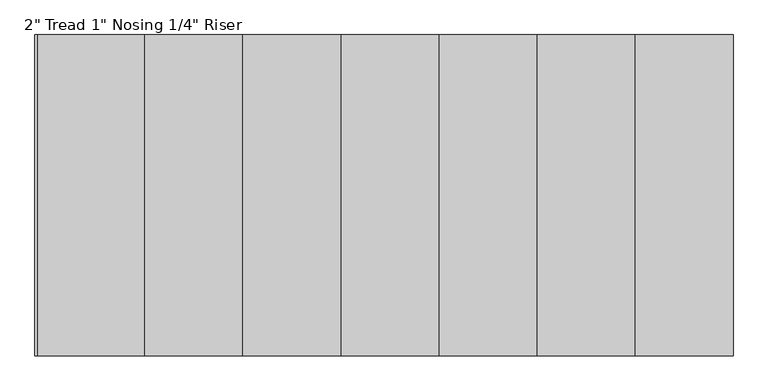
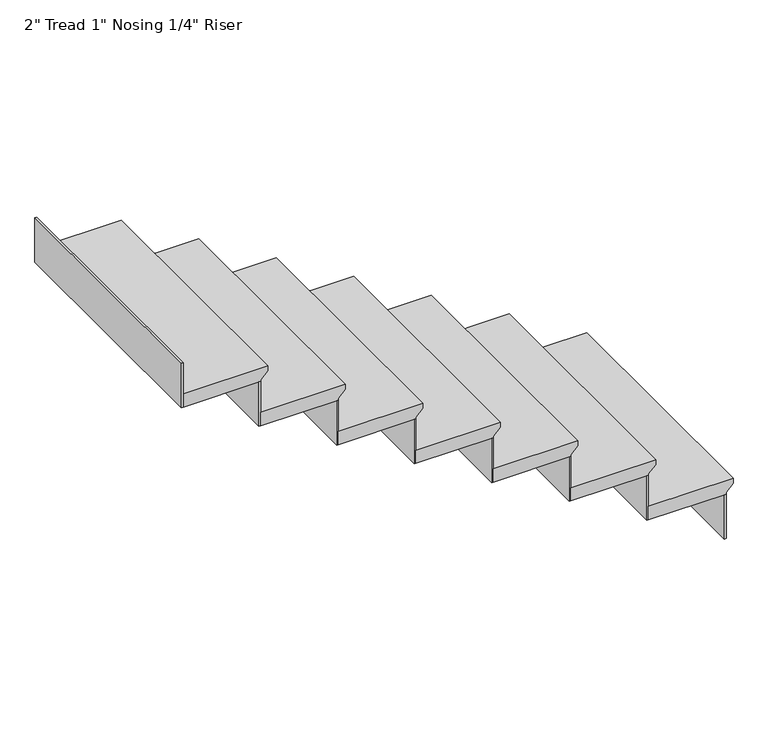
"""IFC4 building model written with IfcOpenShell, lengths in millimetres: stair flight geometry."""

from ifc_helpers import new_model, si_unit, frame, origin, place, context, project, spatial, polyline, outline, extrude, source, transform, mapped, element, save


def stair_flight_2b211656(model_context):
    return source(origin(), model_context, "Body", "SweptSolid", [
        extrude(outline(polyline([(11277.6, 530.5869613), (11277.6, 225.7869613), (11226.8, 225.7869613), (11226.8, 505.1869613), (11233.15, 505.1869613), (11258.55, 530.5869613), (11277.6, 530.5869613)])), frame((0.0, 1135.350634, 0.0), z_axis=(0.0, 1.0, 0.0), x_axis=(0.0, 0.0, 1.0)), (0.0, 0.0, 1.0), 914.4),
        extrude(outline(polyline([(498.8369613, 2049.750634), (505.1869613, 2049.750634), (505.1869613, 1135.350634), (498.8369613, 1135.350634), (498.8369613, 2049.750634)])), frame((0.0, 0.0, 11057.4666667), z_axis=(0.0, 0.0, 1.0), x_axis=(1.0, 0.0, 0.0)), (0.0, 0.0, 1.0), 169.3333333),
        extrude(outline(polyline([(219.4369613, 2049.750634), (225.7869613, 2049.750634), (225.7869613, 1135.350634), (219.4369613, 1135.350634), (219.4369613, 2049.750634)])), frame((0.0, 0.0, 11226.8), z_axis=(0.0, 0.0, 1.0), x_axis=(1.0, 0.0, 0.0)), (0.0, 0.0, 1.0), 169.3333333),
        extrude(outline(polyline([(11446.9333333, 251.1869613), (11446.9333333, -53.6130387), (11396.1333333, -53.6130387), (11396.1333333, 225.7869613), (11402.4833333, 225.7869613), (11427.8833333, 251.1869613), (11446.9333333, 251.1869613)])), frame((0.0, 1135.350634, 0.0), z_axis=(0.0, 1.0, 0.0), x_axis=(0.0, 0.0, 1.0)), (0.0, 0.0, 1.0), 914.4),
        extrude(outline(polyline([(-59.9630387, 2049.750634), (-53.6130387, 2049.750634), (-53.6130387, 1135.350634), (-59.9630387, 1135.350634), (-59.9630387, 2049.750634)])), frame((0.0, 0.0, 11396.1333333), z_axis=(0.0, 0.0, 1.0), x_axis=(1.0, 0.0, 0.0)), (0.0, 0.0, 1.0), 169.3333333),
        extrude(outline(polyline([(11616.2666667, -28.2130387), (11616.2666667, -333.0130387), (11565.4666667, -333.0130387), (11565.4666667, -53.6130387), (11571.8166667, -53.6130387), (11597.2166667, -28.2130387), (11616.2666667, -28.2130387)])), frame((0.0, 1135.350634, 0.0), z_axis=(0.0, 1.0, 0.0), x_axis=(0.0, 0.0, 1.0)), (0.0, 0.0, 1.0), 914.4),
        extrude(outline(polyline([(-339.3630387, 2049.750634), (-333.0130387, 2049.750634), (-333.0130387, 1135.350634), (-339.3630387, 1135.350634), (-339.3630387, 2049.750634)])), frame((0.0, 0.0, 11565.4666667), z_axis=(0.0, 0.0, 1.0), x_axis=(1.0, 0.0, 0.0)), (0.0, 0.0, 1.0), 169.3333333),
        extrude(outline(polyline([(11785.6, -307.6130387), (11785.6, -612.4130387), (11734.8, -612.4130387), (11734.8, -333.0130387), (11741.15, -333.0130387), (11766.55, -307.6130387), (11785.6, -307.6130387)])), frame((0.0, 1135.350634, 0.0), z_axis=(0.0, 1.0, 0.0), x_axis=(0.0, 0.0, 1.0)), (0.0, 0.0, 1.0), 914.4),
        extrude(outline(polyline([(-618.7630387, 2049.750634), (-612.4130387, 2049.750634), (-612.4130387, 1135.350634), (-618.7630387, 1135.350634), (-618.7630387, 2049.750634)])), frame((0.0, 0.0, 11734.8), z_axis=(0.0, 0.0, 1.0), x_axis=(1.0, 0.0, 0.0)), (0.0, 0.0, 1.0), 169.3333333),
        extrude(outline(polyline([(11954.9333333, -587.0130387), (11954.9333333, -891.8130387), (11904.1333333, -891.8130387), (11904.1333333, -612.4130387), (11910.4833333, -612.4130387), (11935.8833333, -587.0130387), (11954.9333333, -587.0130387)])), frame((0.0, 1135.350634, 0.0), z_axis=(0.0, 1.0, 0.0), x_axis=(0.0, 0.0, 1.0)), (0.0, 0.0, 1.0), 914.4),
        extrude(outline(polyline([(-898.1630387, 2049.750634), (-891.8130387, 2049.750634), (-891.8130387, 1135.350634), (-898.1630387, 1135.350634), (-898.1630387, 2049.750634)])), frame((0.0, 0.0, 11904.1333333), z_axis=(0.0, 0.0, 1.0), x_axis=(1.0, 0.0, 0.0)), (0.0, 0.0, 1.0), 169.3333333),
        extrude(outline(polyline([(12124.2666667, -866.4130387), (12124.2666667, -1171.2130387), (12073.4666667, -1171.2130387), (12073.4666667, -891.8130387), (12079.8166667, -891.8130387), (12105.2166667, -866.4130387), (12124.2666667, -866.4130387)])), frame((0.0, 1135.350634, 0.0), z_axis=(0.0, 1.0, 0.0), x_axis=(0.0, 0.0, 1.0)), (0.0, 0.0, 1.0), 914.4),
        extrude(outline(polyline([(-1177.5630387, 2049.750634), (-1171.2130387, 2049.750634), (-1171.2130387, 1135.350634), (-1177.5630387, 1135.350634), (-1177.5630387, 2049.750634)])), frame((0.0, 0.0, 12073.4666667), z_axis=(0.0, 0.0, 1.0), x_axis=(1.0, 0.0, 0.0)), (0.0, 0.0, 1.0), 169.3333333),
        extrude(outline(polyline([(-1456.9630387, 2049.750634), (-1450.6130387, 2049.750634), (-1450.6130387, 1135.350634), (-1456.9630387, 1135.350634), (-1456.9630387, 2049.750634)])), frame((0.0, 0.0, 12242.8), z_axis=(0.0, 0.0, 1.0), x_axis=(1.0, 0.0, 0.0)), (0.0, 0.0, 1.0), 169.3333333),
        extrude(outline(polyline([(12293.6, -1145.8130387), (12293.6, -1450.6130387), (12242.8, -1450.6130387), (12242.8, -1171.2130387), (12249.15, -1171.2130387), (12274.55, -1145.8130387), (12293.6, -1145.8130387)])), frame((0.0, 1135.350634, 0.0), z_axis=(0.0, 1.0, 0.0), x_axis=(0.0, 0.0, 1.0)), (0.0, 0.0, 1.0), 914.4),
    ])


if __name__ == "__main__":
    model = new_model("IFC4")
    model_context = context("Model", 3, world=origin())
    ifc_project = project(units=[si_unit("LENGTHUNIT", "METRE", prefix="MILLI")], contexts=[model_context])
    site = spatial("IfcSite", under=ifc_project)
    building = spatial("IfcBuilding", under=site)
    placement = place(None, origin())
    stair_flight_shape = stair_flight_2b211656(model_context)
    element("IfcStairFlight", 1, ObjectType="2\" Tread 1\" Nosing 1/4\" Riser", at=placement, inside=building, context=model_context, shape_type="MappedRepresentation", body=[
        mapped(stair_flight_shape, transform((0.0, 0.0, 0.0), x_axis=(1.0, 0.0, 0.0), y_axis=(0.0, 1.0, 0.0), z_axis=(0.0, 0.0, 1.0))),
    ])
    save(model, "model.ifc")

# Revit data of these elements
# Element 1 (IfcStairFlight, "2\" Tread 1\" Nosing 1/4\" Riser")
#   Materials on its faces: "BURGUNDY COLOUR"
# Materials
#   "BURGUNDY COLOUR": class "Generic", colour RGB 120 120 120, transparency 0, Cost = 0
